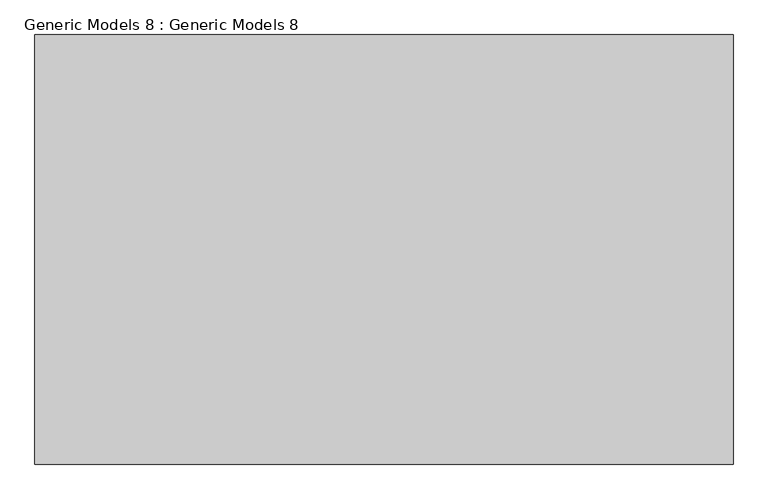
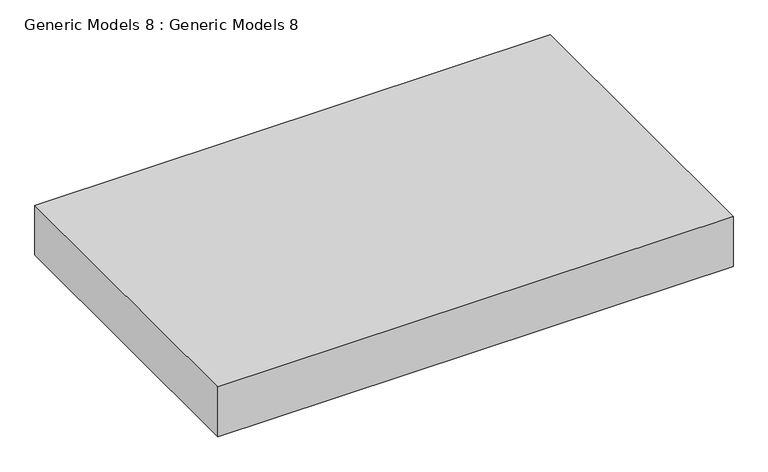
"""IFC4 building model written with IfcOpenShell, lengths in millimetres: proxy geometry, Generic Models 8 : Generic Models 8."""

from ifc_helpers import new_model, si_unit, frame, origin, place, context, project, spatial, polyline, outline, extrude, source, transform, mapped, element, save


def generic_models_8_generic_models_8_7ecb40ae(model_context):
    return source(origin(), model_context, "Body", "SweptSolid", [
        extrude(outline(polyline([(2190.75, -32110.4645004), (2190.75, -31958.0645004), (2190.75, -30776.9645004), (2190.75, -30624.5645004), (2343.15, -30624.5645004), (2343.15, -32110.4645004), (2190.75, -32110.4645004)])), frame((0.0, 20292.3756148, 0.0), z_axis=(0.0, 1.0, 0.0), x_axis=(0.0, 0.0, 1.0)), (0.0, 0.0, 1.0), 914.4),
    ])


if __name__ == "__main__":
    model = new_model("IFC4")
    model_context = context("Model", 3, world=origin())
    ifc_project = project(units=[si_unit("LENGTHUNIT", "METRE", prefix="MILLI")], contexts=[model_context])
    site = spatial("IfcSite", under=ifc_project)
    building = spatial("IfcBuilding", under=site)
    placement = place(None, origin())
    generic_models_8_generic_models_8_shape = generic_models_8_generic_models_8_7ecb40ae(model_context)
    element("IfcBuildingElementProxy", 1, Name="Generic Models 8 : Generic Models 8", ObjectType="Generic Models 8 : Generic Models 8", at=placement, inside=building, context=model_context, shape_type="MappedRepresentation", body=[
        mapped(generic_models_8_generic_models_8_shape, transform((0.0, 0.0, 0.0), x_axis=(1.0, 0.0, 0.0), y_axis=(0.0, 1.0, 0.0), z_axis=(0.0, 0.0, 1.0))),
    ])
    save(model, "model.ifc")
